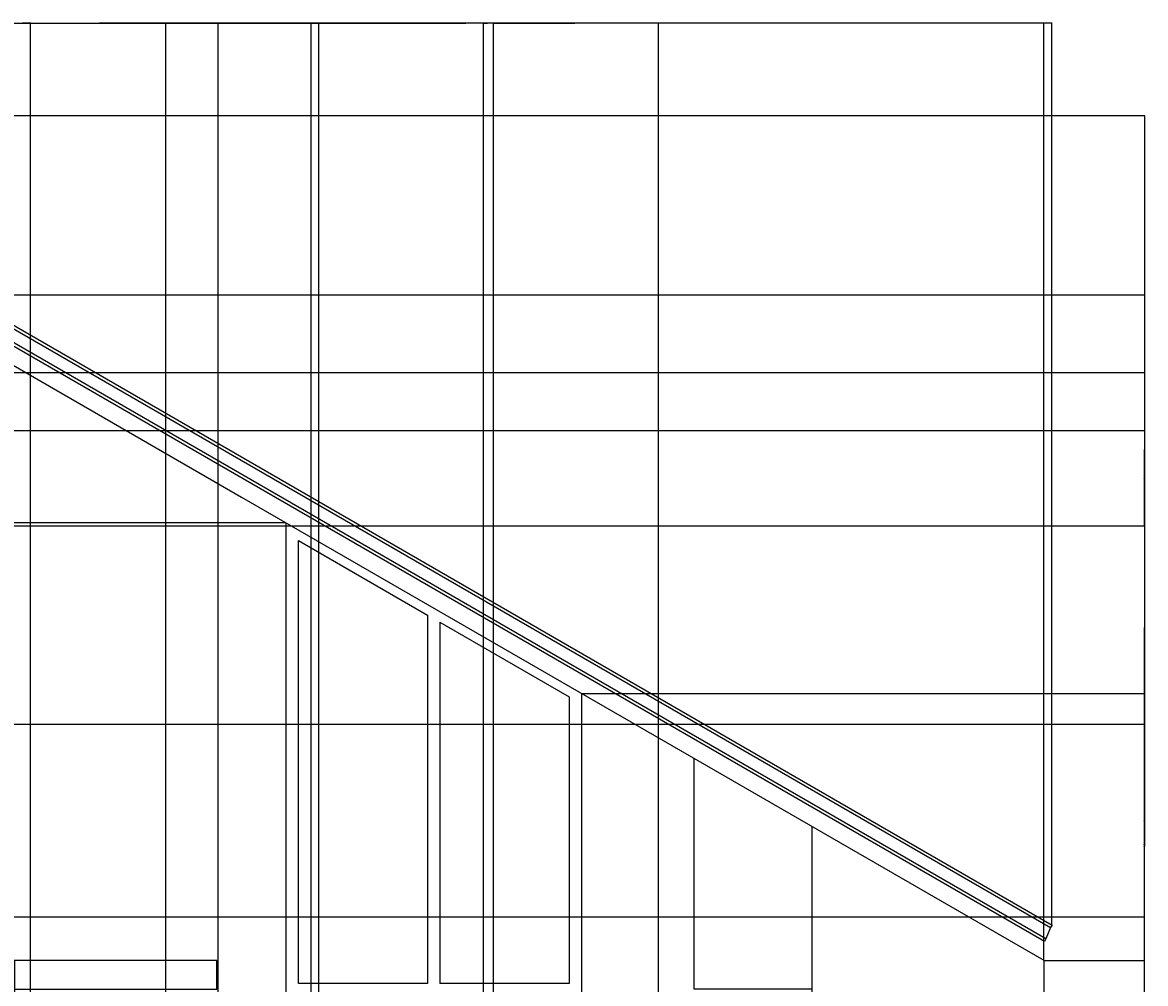
# Model space of a CAD drawing. Units: millimetres. Extents: x 171 to 1599, y 973 to 1509.
# Tile 7 of 7: x 1235 to 1599, y 1196 to 1508. Entities that reach past the tile are written whole.
import ezdxf

# ---------------------------------------------------------------- set-up
doc = ezdxf.new("R2010")
doc.units = ezdxf.units.MM
doc.layers.add('A-ANNO-DIMS', color=2, linetype='Continuous', lineweight=18)
doc.layers.add('A-ELEV', color=7, linetype='Continuous', lineweight=25)
doc.styles.get("Standard").update_dxf_attribs({"font": 'arial.ttf'})
doc.dimstyles.get("Standard").update_dxf_attribs({"dimtxt": 0.18, "dimasz": 0.18, "dimexe": 0.18, "dimexo": 0.0625, "dimgap": 0.09, "dimtad": 0, "dimtih": 1, "dimtoh": 1, "dimdec": 1, "dimzin": 0, "dimdsep": 46, "dimlunit": 3, "dimtxsty": 'Standard', "dimcen": 0.09, "dimadec": 0, "dimazin": 0, "dimtfac": 1, "dimtdec": 1, "dimtofl": 0, "dimtmove": 0, "dimatfit": 3, "dimfxl": 1, "dimtolj": 1, "dimtzin": 0, "dimarcsym": 0})

# ---------------------------------------------------------------- blocks, each defined once
blk = doc.blocks.new('*D1')
at = {"layer": 'A-ANNO-DIMS', "color": 0, "lineweight": -2, "transparency": 16777216}
for p, q in [((980.93, 1194.55), (980.93, 1508.31)), ((981.11, 1508.13), (1274.61, 1508.13)), ((1568.85, 1508.13), (1275.36, 1508.13)), ((1569.03, 1215.31), (1569.03, 1508.31))]:
    blk.add_line(p, q, dxfattribs=at)
at = {"layer": 'A-ANNO-DIMS', "color": 0, "transparency": 16777216}
for points in [[(981.11, 1508.16), (981.11, 1508.1), (980.93, 1508.13)], [(1568.85, 1508.16), (1568.85, 1508.1), (1569.03, 1508.13)]]:
    blk.add_solid(points, dxfattribs=at)
at = {"layer": 'Defpoints', "color": 0, "transparency": 16777216}
for p in [(1569.03, 1508.13), (1569.03, 1215.25), (980.93, 1194.49)]:
    blk.add_point(p, dxfattribs=at)
at = {"layer": 'A-ANNO-DIMS', "color": 0, "transparency": 16777216, "insert": (1274.98, 1508.13), "char_height": 0.18, "attachment_point": 5}
blk.add_mtext('\\A1;588.1', dxfattribs=at)
blk = doc.blocks.new('*D2')
at = {"layer": 'A-ANNO-DIMS', "color": 0, "lineweight": -2, "transparency": 16777216}
for p, q in [((1043.70287, 1478.130098), (1599.212656, 1478.130098)), ((1599.032656, 1477.950098), (1599.032656, 1240.959874)), ((1599.032656, 1003.60965), (1599.032656, 1240.599874)), ((1348.449149, 1003.42965), (1599.212656, 1003.42965))]:
    blk.add_line(p, q, dxfattribs=at)
at = {"layer": 'A-ANNO-DIMS', "color": 0, "transparency": 16777216}
for points in [[(1599.002656, 1477.950098), (1599.062656, 1477.950098), (1599.032656, 1478.130098)], [(1599.002656, 1003.60965), (1599.062656, 1003.60965), (1599.032656, 1003.42965)]]:
    blk.add_solid(points, dxfattribs=at)
at = {"layer": 'Defpoints', "color": 0, "transparency": 16777216}
for p in [(1043.64037, 1478.130098), (1599.032656, 1478.130098), (1348.386649, 1003.42965)]:
    blk.add_point(p, dxfattribs=at)
at = {"layer": 'A-ANNO-DIMS', "color": 0, "transparency": 16777216, "insert": (1599.032656, 1240.779874), "char_height": 0.18, "attachment_point": 5}
blk.add_mtext('\\A1;474.7', dxfattribs=at)
blk = doc.blocks.new('*D42')
at = {"layer": 'A-ANNO-DIMS', "color": 0, "lineweight": -2, "transparency": 16777216}
for p, q in [((1192.02, 1419.99), (1192.02, 1508.31)), ((1192.2, 1508.13), (1378.72, 1508.13)), ((1566.18, 1508.13), (1379.65, 1508.13)), ((1566.36, 1203.87), (1566.36, 1508.31))]:
    blk.add_line(p, q, dxfattribs=at)
at = {"layer": 'A-ANNO-DIMS', "color": 0, "transparency": 16777216}
for points in [[(1192.2, 1508.16), (1192.2, 1508.1), (1192.02, 1508.13)], [(1566.18, 1508.16), (1566.18, 1508.1), (1566.36, 1508.13)]]:
    blk.add_solid(points, dxfattribs=at)
at = {"layer": 'Defpoints', "color": 0, "transparency": 16777216}
for p in [(1566.36, 1508.13), (1192.02, 1419.93), (1566.36, 1203.8)]:
    blk.add_point(p, dxfattribs=at)
at = {"layer": 'A-ANNO-DIMS', "color": 0, "transparency": 16777216, "insert": (1379.19, 1508.13), "char_height": 0.18, "attachment_point": 5}
blk.add_mtext('\\A1;374.34', dxfattribs=at)
blk = doc.blocks.new('*D45')
at = {"layer": 'A-ANNO-DIMS', "color": 0, "lineweight": -2, "transparency": 16777216}
for p, q in [((1064.57, 1394.67), (1599.21, 1394.67)), ((1599.03, 1394.49), (1599.03, 1369.95)), ((1599.03, 1345.05), (1599.03, 1369.59)), ((1105.88, 1344.87), (1599.21, 1344.87))]:
    blk.add_line(p, q, dxfattribs=at)
at = {"layer": 'A-ANNO-DIMS', "color": 0, "transparency": 16777216}
for points in [[(1599, 1394.49), (1599.06, 1394.49), (1599.03, 1394.67)], [(1599, 1345.05), (1599.06, 1345.05), (1599.03, 1344.87)]]:
    blk.add_solid(points, dxfattribs=at)
at = {"layer": 'Defpoints', "color": 0, "transparency": 16777216}
for p in [(1064.5, 1394.67), (1105.82, 1344.87), (1599.03, 1344.87)]:
    blk.add_point(p, dxfattribs=at)
at = {"layer": 'A-ANNO-DIMS', "color": 0, "transparency": 16777216, "insert": (1599.03, 1369.77), "char_height": 0.18, "attachment_point": 5}
blk.add_mtext('\\A1;49.80', dxfattribs=at)
blk = doc.blocks.new('*D46')
at = {"layer": 'A-ANNO-DIMS', "color": 0, "lineweight": -2, "transparency": 16777216}
for p, q in [((1198.36, 1375.85), (1599.21, 1375.85)), ((1599.03, 1375.67), (1599.03, 1360.54)), ((1599.03, 1345.05), (1599.03, 1360.18)), ((1185.8, 1344.87), (1599.21, 1344.87))]:
    blk.add_line(p, q, dxfattribs=at)
at = {"layer": 'A-ANNO-DIMS', "color": 0, "transparency": 16777216}
for points in [[(1599, 1375.67), (1599.06, 1375.67), (1599.03, 1375.85)], [(1599, 1345.05), (1599.06, 1345.05), (1599.03, 1344.87)]]:
    blk.add_solid(points, dxfattribs=at)
at = {"layer": 'Defpoints', "color": 0, "transparency": 16777216}
for p in [(1198.29, 1375.85), (1599.03, 1375.85), (1185.73, 1344.87)]:
    blk.add_point(p, dxfattribs=at)
at = {"layer": 'A-ANNO-DIMS', "color": 0, "transparency": 16777216, "insert": (1599.03, 1360.36), "char_height": 0.18, "attachment_point": 5}
blk.add_mtext('\\A1;30.976', dxfattribs=at)
blk = doc.blocks.new('*D47')
at = {"layer": 'A-ANNO-DIMS', "color": 0, "lineweight": -2, "transparency": 16777216}
for p, q in [((1192.08, 1419.93), (1599.21, 1419.93)), ((1599.03, 1419.75), (1599.03, 1312.05)), ((1599.03, 1203.98), (1599.03, 1311.68)), ((1566.42, 1203.8), (1599.21, 1203.8))]:
    blk.add_line(p, q, dxfattribs=at)
at = {"layer": 'A-ANNO-DIMS', "color": 0, "transparency": 16777216}
for points in [[(1599, 1419.75), (1599.06, 1419.75), (1599.03, 1419.93)], [(1599, 1203.98), (1599.06, 1203.98), (1599.03, 1203.8)]]:
    blk.add_solid(points, dxfattribs=at)
at = {"layer": 'Defpoints', "color": 0, "transparency": 16777216}
for p in [(1192.02, 1419.93), (1566.36, 1203.8), (1599.03, 1203.8)]:
    blk.add_point(p, dxfattribs=at)
at = {"layer": 'A-ANNO-DIMS', "color": 0, "transparency": 16777216, "insert": (1599.03, 1311.87), "char_height": 0.18, "attachment_point": 5}
blk.add_mtext('\\A1;216.13', dxfattribs=at)
blk = doc.blocks.new('*D54')
at = {"layer": 'A-ANNO-DIMS', "color": 0, "lineweight": -2, "transparency": 16777216}
for p, q in [((1232.1, 1203.73), (1232.1, 973.25)), ((1320.32, 1192.2), (1320.32, 973.25)), ((1232.28, 973.43), (1275.82, 973.43)), ((1320.14, 973.43), (1276.6, 973.43))]:
    blk.add_line(p, q, dxfattribs=at)
at = {"layer": 'A-ANNO-DIMS', "color": 0, "transparency": 16777216}
for points in [[(1232.28, 973.46), (1232.28, 973.4), (1232.1, 973.43)], [(1320.14, 973.46), (1320.14, 973.4), (1320.32, 973.43)]]:
    blk.add_solid(points, dxfattribs=at)
at = {"layer": 'Defpoints', "color": 0, "transparency": 16777216}
for p in [(1232.1, 1203.79), (1320.32, 1192.27), (1320.32, 973.43)]:
    blk.add_point(p, dxfattribs=at)
at = {"layer": 'A-ANNO-DIMS', "color": 0, "transparency": 16777216, "insert": (1276.21, 973.43), "char_height": 0.18, "attachment_point": 5}
blk.add_mtext('\\A1;88.22', dxfattribs=at)
blk = doc.blocks.new('*D60')
at = {"layer": 'A-ANNO-DIMS', "color": 0, "lineweight": -2, "transparency": 16777216}
for p, q in [((1566.36, 1203.74), (1566.36, 973.25)), ((1491.01, 1194.43), (1491.01, 973.25)), ((1491.19, 973.43), (1528.29, 973.43)), ((1566.18, 973.43), (1529.08, 973.43))]:
    blk.add_line(p, q, dxfattribs=at)
at = {"layer": 'A-ANNO-DIMS', "color": 0, "transparency": 16777216}
for points in [[(1491.19, 973.46), (1491.19, 973.4), (1491.01, 973.43)], [(1566.18, 973.46), (1566.18, 973.4), (1566.36, 973.43)]]:
    blk.add_solid(points, dxfattribs=at)
at = {"layer": 'Defpoints', "color": 0, "transparency": 16777216}
for p in [(1566.36, 1203.8), (1491.01, 1194.49), (1566.36, 973.43)]:
    blk.add_point(p, dxfattribs=at)
at = {"layer": 'A-ANNO-DIMS', "color": 0, "transparency": 16777216, "insert": (1528.69, 973.43), "char_height": 0.18, "attachment_point": 5}
blk.add_mtext('\\A1;75.35', dxfattribs=at)
blk = doc.blocks.new('*D61')
at = {"layer": 'A-ANNO-DIMS', "color": 0, "lineweight": -2, "transparency": 16777216}
for p, q in [((1320.26, 1345.85), (950.75, 1345.85)), ((950.93, 1345.67), (950.93, 1269.24)), ((950.93, 1192.45), (950.93, 1268.88)), ((1320.26, 1192.27), (950.75, 1192.27))]:
    blk.add_line(p, q, dxfattribs=at)
at = {"layer": 'A-ANNO-DIMS', "color": 0, "transparency": 16777216}
for points in [[(950.9, 1345.67), (950.96, 1345.67), (950.93, 1345.85)], [(950.9, 1192.45), (950.96, 1192.45), (950.93, 1192.27)]]:
    blk.add_solid(points, dxfattribs=at)
at = {"layer": 'Defpoints', "color": 0, "transparency": 16777216}
for p in [(950.93, 1345.85), (1320.32, 1345.85), (1320.32, 1192.27)]:
    blk.add_point(p, dxfattribs=at)
at = {"layer": 'A-ANNO-DIMS', "color": 0, "transparency": 16777216, "insert": (950.93, 1269.06), "char_height": 0.18, "attachment_point": 5}
blk.add_mtext('\\A1;153.59', dxfattribs=at)
blk = doc.blocks.new('*D62')
at = {"layer": 'A-ANNO-DIMS', "color": 0, "lineweight": -2, "transparency": 16777216}
for p, q in [((1416.28, 1290.48), (1599.21, 1290.48)), ((1599.03, 1290.3), (1599.03, 1241.56)), ((1599.03, 1192.45), (1599.03, 1241.19)), ((1416.28, 1192.27), (1599.21, 1192.27))]:
    blk.add_line(p, q, dxfattribs=at)
at = {"layer": 'A-ANNO-DIMS', "color": 0, "transparency": 16777216}
for points in [[(1599, 1290.3), (1599.06, 1290.3), (1599.03, 1290.48)], [(1599, 1192.45), (1599.06, 1192.45), (1599.03, 1192.27)]]:
    blk.add_solid(points, dxfattribs=at)
at = {"layer": 'Defpoints', "color": 0, "transparency": 16777216}
for p in [(1416.22, 1290.48), (1599.03, 1290.48), (1416.22, 1192.27)]:
    blk.add_point(p, dxfattribs=at)
at = {"layer": 'A-ANNO-DIMS', "color": 0, "transparency": 16777216, "insert": (1599.03, 1241.38), "char_height": 0.18, "attachment_point": 5}
blk.add_mtext('\\A1;98.22', dxfattribs=at)
blk = doc.blocks.new('*D63')
at = {"layer": 'A-ANNO-DIMS', "color": 0, "lineweight": -2, "transparency": 16777216}
for p, q in [((1181.8, 1280.52), (1599.21, 1280.52)), ((1599.03, 1280.34), (1599.03, 1249.38)), ((1599.03, 1218.05), (1599.03, 1249.01)), ((1185.8, 1217.87), (1599.21, 1217.87))]:
    blk.add_line(p, q, dxfattribs=at)
at = {"layer": 'A-ANNO-DIMS', "color": 0, "transparency": 16777216}
for points in [[(1599, 1280.34), (1599.06, 1280.34), (1599.03, 1280.52)], [(1599, 1218.05), (1599.06, 1218.05), (1599.03, 1217.87)]]:
    blk.add_solid(points, dxfattribs=at)
at = {"layer": 'Defpoints', "color": 0, "transparency": 16777216}
for p in [(1181.73, 1280.52), (1599.03, 1280.52), (1185.73, 1217.87)]:
    blk.add_point(p, dxfattribs=at)
at = {"layer": 'A-ANNO-DIMS', "color": 0, "transparency": 16777216, "insert": (1599.03, 1249.2), "char_height": 0.18, "attachment_point": 5}
blk.add_mtext('\\A1;62.66', dxfattribs=at)
blk = doc.blocks.new('*D73')
at = {"layer": 'A-ANNO-DIMS', "color": 0, "lineweight": -2, "transparency": 16777216}
for p, q in [((1231.46, 1114.32), (1231.46, 1508.31)), ((1231.64, 1508.13), (1234.06, 1508.13)), ((1237.13, 1508.13), (1234.71, 1508.13)), ((1237.31, 1162.35), (1237.31, 1508.31))]:
    blk.add_line(p, q, dxfattribs=at)
at = {"layer": 'A-ANNO-DIMS', "color": 0, "transparency": 16777216}
for points in [[(1231.64, 1508.16), (1231.64, 1508.1), (1231.46, 1508.13)], [(1237.13, 1508.16), (1237.13, 1508.1), (1237.31, 1508.13)]]:
    blk.add_solid(points, dxfattribs=at)
at = {"layer": 'Defpoints', "color": 0, "transparency": 16777216}
for p in [(1237.31, 1508.13), (1237.31, 1162.29), (1231.46, 1114.25)]:
    blk.add_point(p, dxfattribs=at)
at = {"layer": 'A-ANNO-DIMS', "color": 0, "transparency": 16777216, "insert": (1234.38, 1508.13), "char_height": 0.18, "attachment_point": 5}
blk.add_mtext('\\A1;5.85', dxfattribs=at)
blk = doc.blocks.new('*D74')
at = {"layer": 'A-ANNO-DIMS', "color": 0, "lineweight": -2, "transparency": 16777216}
for p, q in [((1237.31, 1162.35), (1237.31, 1508.31)), ((1237.49, 1508.13), (1258.88, 1508.13)), ((1281.06, 1508.13), (1259.67, 1508.13)), ((1281.24, 1162.35), (1281.24, 1508.31))]:
    blk.add_line(p, q, dxfattribs=at)
at = {"layer": 'A-ANNO-DIMS', "color": 0, "transparency": 16777216}
for points in [[(1237.49, 1508.16), (1237.49, 1508.1), (1237.31, 1508.13)], [(1281.06, 1508.16), (1281.06, 1508.1), (1281.24, 1508.13)]]:
    blk.add_solid(points, dxfattribs=at)
at = {"layer": 'Defpoints', "color": 0, "transparency": 16777216}
for p in [(1281.24, 1508.13), (1237.31, 1162.29), (1281.24, 1162.29)]:
    blk.add_point(p, dxfattribs=at)
at = {"layer": 'A-ANNO-DIMS', "color": 0, "transparency": 16777216, "insert": (1259.27, 1508.13), "char_height": 0.18, "attachment_point": 5}
blk.add_mtext('\\A1;43.93', dxfattribs=at)
blk = doc.blocks.new('*D75')
at = {"layer": 'A-ANNO-DIMS', "color": 0, "lineweight": -2, "transparency": 16777216}
for p, q in [((1281.24, 1162.35), (1281.24, 1508.31)), ((1281.42, 1508.13), (1289.28, 1508.13)), ((1298.06, 1508.13), (1290.19, 1508.13)), ((1298.24, 1177.93), (1298.24, 1508.31))]:
    blk.add_line(p, q, dxfattribs=at)
at = {"layer": 'A-ANNO-DIMS', "color": 0, "transparency": 16777216}
for points in [[(1281.42, 1508.16), (1281.42, 1508.1), (1281.24, 1508.13)], [(1298.06, 1508.16), (1298.06, 1508.1), (1298.24, 1508.13)]]:
    blk.add_solid(points, dxfattribs=at)
at = {"layer": 'Defpoints', "color": 0, "transparency": 16777216}
for p in [(1298.24, 1508.13), (1298.24, 1177.87), (1281.24, 1162.29)]:
    blk.add_point(p, dxfattribs=at)
at = {"layer": 'A-ANNO-DIMS', "color": 0, "transparency": 16777216, "insert": (1289.74, 1508.13), "char_height": 0.18, "attachment_point": 5}
blk.add_mtext('\\A1;16.995', dxfattribs=at)
blk = doc.blocks.new('*D76')
at = {"layer": 'A-ANNO-DIMS', "color": 0, "lineweight": -2, "transparency": 16777216}
for p, q in [((1298.24, 1177.93), (1298.24, 1508.31)), ((1298.42, 1508.13), (1312.96, 1508.13)), ((1328.29, 1508.13), (1313.75, 1508.13)), ((1328.47, 1082.3), (1328.47, 1508.31))]:
    blk.add_line(p, q, dxfattribs=at)
at = {"layer": 'A-ANNO-DIMS', "color": 0, "transparency": 16777216}
for points in [[(1298.42, 1508.16), (1298.42, 1508.1), (1298.24, 1508.13)], [(1328.29, 1508.16), (1328.29, 1508.1), (1328.47, 1508.13)]]:
    blk.add_solid(points, dxfattribs=at)
at = {"layer": 'Defpoints', "color": 0, "transparency": 16777216}
for p in [(1328.47, 1508.13), (1298.24, 1177.87), (1328.47, 1082.23)]:
    blk.add_point(p, dxfattribs=at)
at = {"layer": 'A-ANNO-DIMS', "color": 0, "transparency": 16777216, "insert": (1313.36, 1508.13), "char_height": 0.18, "attachment_point": 5}
blk.add_mtext('\\A1;30.24', dxfattribs=at)
blk = doc.blocks.new('*D77')
at = {"layer": 'A-ANNO-DIMS', "color": 0, "lineweight": -2, "transparency": 16777216}
for p, q in [((1328.47, 1082.3), (1328.47, 1508.31)), ((1328.65, 1508.13), (1329.29, 1508.13)), ((1330.72, 1508.13), (1330.08, 1508.13)), ((1330.9, 1176.81), (1330.9, 1508.31))]:
    blk.add_line(p, q, dxfattribs=at)
at = {"layer": 'A-ANNO-DIMS', "color": 0, "transparency": 16777216}
for points in [[(1328.65, 1508.16), (1328.65, 1508.1), (1328.47, 1508.13)], [(1330.72, 1508.16), (1330.72, 1508.1), (1330.9, 1508.13)]]:
    blk.add_solid(points, dxfattribs=at)
at = {"layer": 'Defpoints', "color": 0, "transparency": 16777216}
for p in [(1330.9, 1508.13), (1330.9, 1176.74), (1328.47, 1082.23)]:
    blk.add_point(p, dxfattribs=at)
at = {"layer": 'A-ANNO-DIMS', "color": 0, "transparency": 16777216, "insert": (1329.69, 1508.13), "char_height": 0.18, "attachment_point": 5}
blk.add_mtext('\\A1;2.423', dxfattribs=at)
blk = doc.blocks.new('*D78')
at = {"layer": 'A-ANNO-DIMS', "color": 0, "lineweight": -2, "transparency": 16777216}
for p, q in [((1330.9, 1176.81), (1330.9, 1508.31)), ((1331.08, 1508.13), (1357.29, 1508.13)), ((1384.29, 1508.13), (1358.08, 1508.13)), ((1384.47, 1172.81), (1384.47, 1508.31))]:
    blk.add_line(p, q, dxfattribs=at)
at = {"layer": 'A-ANNO-DIMS', "color": 0, "transparency": 16777216}
for points in [[(1331.08, 1508.16), (1331.08, 1508.1), (1330.9, 1508.13)], [(1384.29, 1508.16), (1384.29, 1508.1), (1384.47, 1508.13)]]:
    blk.add_solid(points, dxfattribs=at)
at = {"layer": 'Defpoints', "color": 0, "transparency": 16777216}
for p in [(1384.47, 1508.13), (1330.9, 1176.74), (1384.47, 1172.74)]:
    blk.add_point(p, dxfattribs=at)
at = {"layer": 'A-ANNO-DIMS', "color": 0, "transparency": 16777216, "insert": (1357.69, 1508.13), "char_height": 0.18, "attachment_point": 5}
blk.add_mtext('\\A1;53.58', dxfattribs=at)
blk = doc.blocks.new('*D79')
at = {"layer": 'A-ANNO-DIMS', "color": 0, "lineweight": -2, "transparency": 16777216}
for p, q in [((1384.47, 1172.81), (1384.47, 1508.31)), ((1384.65, 1508.13), (1385.69, 1508.13)), ((1387.52, 1508.13), (1386.48, 1508.13)), ((1387.7, 1172.81), (1387.7, 1508.31))]:
    blk.add_line(p, q, dxfattribs=at)
at = {"layer": 'A-ANNO-DIMS', "color": 0, "transparency": 16777216}
for points in [[(1384.65, 1508.16), (1384.65, 1508.1), (1384.47, 1508.13)], [(1387.52, 1508.16), (1387.52, 1508.1), (1387.7, 1508.13)]]:
    blk.add_solid(points, dxfattribs=at)
at = {"layer": 'Defpoints', "color": 0, "transparency": 16777216}
for p in [(1387.7, 1508.13), (1384.47, 1172.74), (1387.7, 1172.74)]:
    blk.add_point(p, dxfattribs=at)
at = {"layer": 'A-ANNO-DIMS', "color": 0, "transparency": 16777216, "insert": (1386.09, 1508.13), "char_height": 0.18, "attachment_point": 5}
blk.add_mtext('\\A1;3.224', dxfattribs=at)
blk = doc.blocks.new('*D80')
at = {"layer": 'A-ANNO-DIMS', "color": 0, "lineweight": -2, "transparency": 16777216}
for p, q in [((1387.7, 1172.81), (1387.7, 1508.31)), ((1387.88, 1508.13), (1414.09, 1508.13)), ((1441.1, 1508.13), (1414.88, 1508.13)), ((1441.28, 1176.81), (1441.28, 1508.31))]:
    blk.add_line(p, q, dxfattribs=at)
at = {"layer": 'A-ANNO-DIMS', "color": 0, "transparency": 16777216}
for points in [[(1387.88, 1508.16), (1387.88, 1508.1), (1387.7, 1508.13)], [(1441.1, 1508.16), (1441.1, 1508.1), (1441.28, 1508.13)]]:
    blk.add_solid(points, dxfattribs=at)
at = {"layer": 'Defpoints', "color": 0, "transparency": 16777216}
for p in [(1441.28, 1508.13), (1441.28, 1176.74), (1387.7, 1172.74)]:
    blk.add_point(p, dxfattribs=at)
at = {"layer": 'A-ANNO-DIMS', "color": 0, "transparency": 16777216, "insert": (1414.49, 1508.13), "char_height": 0.18, "attachment_point": 5}
blk.add_mtext('\\A1;53.58', dxfattribs=at)

msp = doc.modelspace()

# ---------------------------------------------------------------- linework, layer by layer
at = {"layer": 'A-ELEV'}
for p, q in [((1324.3201, 1340.0799), (1366.2709, 1315.8596)), ((1366.2709, 1315.8596), (1366.2709, 1196.267)), ((1370.2709, 1313.5502), (1370.2709, 1196.267)), ((1370.2709, 1313.5502), (1412.2216, 1289.3299))]:
    msp.add_line(p, q, dxfattribs=at)
for points in [[(1200.1219, 1427.1523), (1200.594, 1427.97), (1569.0327, 1215.2519), (1568.5605, 1214.4341), (1566.9934, 1210.7354), (1566.5754, 1209.8864), (1197.176, 1423.1592), (1197.3929, 1423.034), (1192.0162, 1419.9297), (1305.8587, 1354.2027), (1566.3585, 1203.8031), (1566.3585, 1210.0116)], [(1566.9934, 1210.7354), (1197.7023, 1423.9457), (1200.1219, 1427.1523), (1568.5605, 1214.4341)], [(1416.2216, 1290.4846), (1416.2216, 1192.267), (1320.3201, 1192.267), (1320.3201, 1345.8534)], [(1366.2709, 1196.267), (1324.3201, 1196.267), (1324.3201, 1340.0799)], [(1412.2216, 1289.3299), (1412.2216, 1196.267), (1370.2709, 1196.267)], [(1491.0132, 1247.3037), (1491.0132, 1194.488), (1452.8572, 1194.488), (1452.8572, 1269.3331)], [(980.9303, 1194.488), (1297.8374, 1194.488), (1297.8374, 1203.7941), (980.9303, 1203.7941)]]:
    msp.add_lwpolyline(points, dxfattribs=at)

# ---------------------------------------------------------------- dimensions: what is measured, and where the dimension line sits
at = {"layer": 'A-ANNO-DIMS'}
for base, p1, p2, override, picture, middle in [((1569.0327, 1508.1301), (980.9303, 1194.488), (1569.0327, 1215.2519), {"dimdec": 1, "dimlfac": 1, "dimrnd": 0, "dimzin": 0, "dimdsep": 46, "dimlunit": 2}, '*D1', (1274.9815, 1508.1301)), ((1566.3585, 1508.1301), (1192.0162, 1419.9297), (1566.3585, 1203.8031), {"dimdec": 2, "dimlfac": 1, "dimrnd": 0, "dimzin": 0, "dimdsep": 46, "dimlunit": 2}, '*D42', (1379.1873, 1508.1301)), ((1237.3083, 1508.1301), (1231.4586, 1114.2546), (1237.3083, 1162.2854), {"dimdec": 2, "dimlfac": 1, "dimrnd": 0, "dimzin": 0, "dimdsep": 46, "dimlunit": 2}, '*D73', (1234.3834, 1508.1301)), ((1281.2416, 1508.1301), (1237.3083, 1162.2854), (1281.2416, 1162.2854), {"dimdec": 2, "dimlfac": 1, "dimrnd": 0, "dimzin": 0, "dimdsep": 46, "dimlunit": 2}, '*D74', (1259.275, 1508.1301)), ((1298.2363, 1508.1301), (1281.2416, 1162.2854), (1298.2363, 1177.8722), {"dimdec": 3, "dimlfac": 1, "dimrnd": 0, "dimzin": 0, "dimdsep": 46, "dimlunit": 2}, '*D75', (1289.739, 1508.1301)), ((1328.4737, 1508.1301), (1298.2363, 1177.8722), (1328.4737, 1082.2327), {"dimdec": 2, "dimlfac": 1, "dimrnd": 0, "dimzin": 0, "dimdsep": 46, "dimlunit": 2}, '*D76', (1313.355, 1508.1301)), ((1330.8966, 1508.1301), (1328.4737, 1082.2327), (1330.8966, 1176.7441), {"dimdec": 3, "dimlfac": 1, "dimrnd": 0, "dimzin": 0, "dimdsep": 46, "dimlunit": 2}, '*D77', (1329.6852, 1508.1301)), ((1384.4743, 1508.1301), (1330.8966, 1176.7441), (1384.4743, 1172.7441), {"dimdec": 2, "dimlfac": 1, "dimrnd": 0, "dimzin": 0, "dimdsep": 46, "dimlunit": 2}, '*D78', (1357.6855, 1508.1301)), ((1387.6984, 1508.1301), (1384.4743, 1172.7441), (1387.6984, 1172.7441), {"dimdec": 3, "dimlfac": 1, "dimrnd": 0, "dimzin": 0, "dimdsep": 46, "dimlunit": 2}, '*D79', (1386.0864, 1508.1301)), ((1441.2762, 1508.1301), (1387.6984, 1172.7441), (1441.2762, 1176.7441), {"dimdec": 2, "dimlfac": 1, "dimrnd": 0, "dimzin": 0, "dimdsep": 46, "dimlunit": 2}, '*D80', (1414.4873, 1508.1301)), ((1320.3201, 973.4297), (1232.0993, 1203.7941), (1320.3201, 1192.267), {"dimdec": 2, "dimlfac": 1, "dimrnd": 0, "dimzin": 0, "dimdsep": 46, "dimlunit": 2}, '*D54', (1276.2097, 973.4297)), ((1566.3585, 973.4297), (1491.0132, 1194.488), (1566.3585, 1203.8031), {"dimdec": 2, "dimlfac": 1, "dimrnd": 0, "dimzin": 0, "dimdsep": 46, "dimlunit": 2}, '*D60', (1528.6858, 973.4297))]:
    dim = msp.add_linear_dim(base=base, p1=p1, p2=p2, dimstyle='Standard', override=override, dxfattribs=at)
    dim.commit()
    dim.dimension.update_dxf_attribs({"geometry": picture, "text_midpoint": middle})
for base, p1, p2, override, picture, middle in [((1599.0327, 1478.1301), (1348.3866, 1003.4297), (1043.6404, 1478.1301), {"dimdec": 1, "dimlfac": 1, "dimrnd": 0, "dimzin": 0, "dimdsep": 46, "dimlunit": 2}, '*D2', (1599.0327, 1240.7799)), ((1599.0327, 1203.8031), (1192.0162, 1419.9297), (1566.3585, 1203.8031), {"dimdec": 2, "dimlfac": 1, "dimrnd": 0, "dimzin": 0, "dimdsep": 46, "dimlunit": 2}, '*D47', (1599.0327, 1311.8664)), ((1599.0327, 1344.8717), (1064.505, 1394.6687), (1105.8176, 1344.8717), {"dimdec": 2, "dimlfac": 1, "dimrnd": 0, "dimzin": 0, "dimdsep": 46, "dimlunit": 2}, '*D45', (1599.0327, 1369.7702)), ((1599.0327, 1375.8481), (1185.7346, 1344.8717), (1198.2939, 1375.8481), {"dimdec": 3, "dimlfac": 1, "dimrnd": 0, "dimzin": 0, "dimdsep": 46, "dimlunit": 2}, '*D46', (1599.0327, 1360.3599)), ((950.9303, 1345.8534), (1320.3201, 1192.267), (1320.3201, 1345.8534), {"dimdec": 2, "dimlfac": 1, "dimrnd": 0, "dimzin": 0, "dimdsep": 46, "dimlunit": 2}, '*D61', (950.9303, 1269.0602)), ((1599.0327, 1290.4846), (1416.2216, 1192.267), (1416.2216, 1290.4846), {"dimdec": 2, "dimlfac": 1, "dimrnd": 0, "dimzin": 0, "dimdsep": 46, "dimlunit": 2}, '*D62', (1599.0327, 1241.3758)), ((1599.0327, 1280.5242), (1185.7346, 1217.867), (1181.7346, 1280.5242), {"dimdec": 2, "dimlfac": 1, "dimrnd": 0, "dimzin": 0, "dimdsep": 46, "dimlunit": 2}, '*D63', (1599.0327, 1249.1956))]:
    dim = msp.add_linear_dim(base=base, p1=p1, p2=p2, angle=90, dimstyle='Standard', override=override, dxfattribs=at)
    dim.commit()
    dim.dimension.update_dxf_attribs({"geometry": picture, "text_midpoint": middle})

doc.saveas('drawing.dxf')
